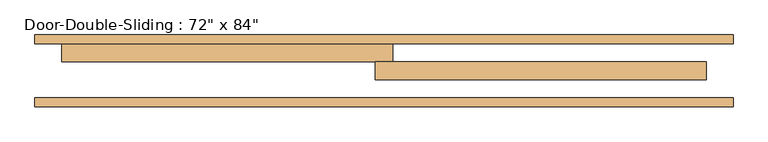
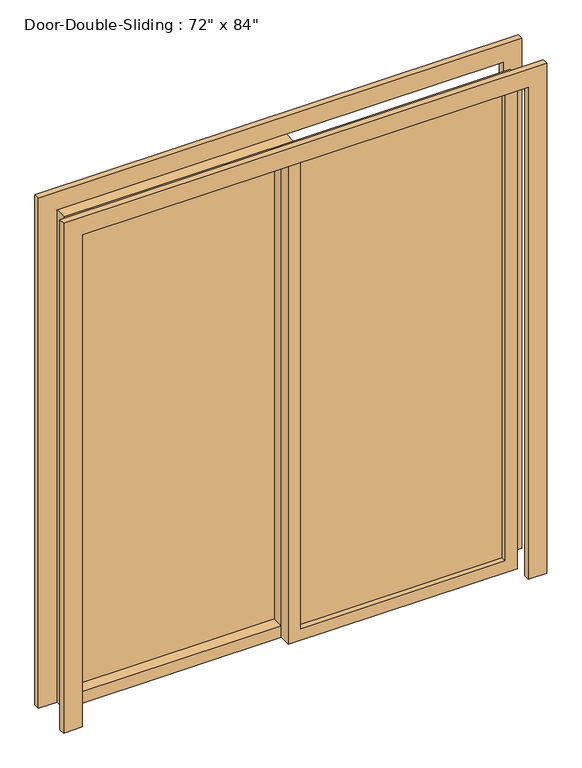
"""IFC4 building model written with IfcOpenShell, lengths in millimetres: door geometry."""

from ifc_helpers import new_model, si_unit, frame, origin, place, context, project, spatial, polyline, outline, extrude, source, transform, mapped, element, save


def door_b43bda57(model_context):
    return source(origin(), model_context, "Body", "SweptSolid", [
        extrude(outline(polyline([(0.0, -990.6), (0.0, -914.4), (2133.6, -914.4), (2133.6, 914.4), (0.0, 914.4), (0.0, 990.6), (2209.8, 990.6), (2209.8, -990.6), (0.0, -990.6)])), frame((0.0, 25.4, 0.0), z_axis=(0.0, 1.0, 0.0), x_axis=(0.0, 0.0, 1.0)), (0.0, 0.0, 1.0), 25.4),
        extrude(outline(polyline([(0.0, 990.6), (2209.8, 990.6), (2209.8, -990.6), (0.0, -990.6), (0.0, -914.4), (2133.6, -914.4), (2133.6, 914.4), (0.0, 914.4), (0.0, 990.6)])), frame((0.0, 203.2, 0.0), z_axis=(0.0, 1.0, 0.0), x_axis=(0.0, 0.0, 1.0)), (0.0, 0.0, 1.0), 25.4),
        extrude(outline(polyline([(2133.6, -25.4), (0.0, -25.4), (0.0, 914.4), (2133.6, 914.4), (2133.6, -25.4)]), holes=[polyline([(2082.8, 25.4), (2082.8, 863.6), (50.8, 863.6), (50.8, 25.4), (2082.8, 25.4)])]), frame((0.0, 101.6, 0.0), z_axis=(0.0, 1.0, 0.0), x_axis=(0.0, 0.0, 1.0)), (0.0, 0.0, 1.0), 50.8),
        extrude(outline(polyline([(2133.6, 25.4), (2133.6, -914.4), (0.0, -914.4), (0.0, 25.4), (2133.6, 25.4)]), holes=[polyline([(2082.8, -25.4), (50.8, -25.4), (50.8, -863.6), (2082.8, -863.6), (2082.8, -25.4)])]), frame((0.0, 152.4, 0.0), z_axis=(0.0, 1.0, 0.0), x_axis=(0.0, 0.0, 1.0)), (0.0, 0.0, 1.0), 50.8),
        extrude(outline(polyline([(25.4, 130.175), (863.6, 130.175), (863.6, 123.825), (25.4, 123.825), (25.4, 130.175)])), frame((0.0, 0.0, 50.8), z_axis=(0.0, 0.0, 1.0), x_axis=(1.0, 0.0, 0.0)), (0.0, 0.0, 1.0), 2032.0),
        extrude(outline(polyline([(-25.4, 200.025), (-863.6, 200.025), (-863.6, 206.375), (-25.4, 206.375), (-25.4, 200.025)])), frame((0.0, 0.0, 50.8), z_axis=(0.0, 0.0, 1.0), x_axis=(1.0, 0.0, 0.0)), (0.0, 0.0, 1.0), 2032.0),
    ])


if __name__ == "__main__":
    model = new_model("IFC4")
    model_context = context("Model", 3, world=origin())
    ifc_project = project(units=[si_unit("LENGTHUNIT", "METRE", prefix="MILLI")], contexts=[model_context])
    site = spatial("IfcSite", under=ifc_project)
    building = spatial("IfcBuilding", under=site)
    placement = place(None, origin())
    door_shape = door_b43bda57(model_context)
    element("IfcDoor", 1, ObjectType="Door-Double-Sliding : 72\" x 84\"", at=placement, inside=building, context=model_context, shape_type="MappedRepresentation", body=[
        mapped(door_shape, transform((0.0, 0.0, 0.0), x_axis=(1.0, 0.0, 0.0), y_axis=(0.0, 1.0, 0.0), z_axis=(0.0, 0.0, 1.0))),
    ])
    save(model, "model.ifc")

# Revit data of these elements
# Type "Door-Double-Sliding : 72\" x 84\""
#   Type Mark = "9"
#   Construction Type Id = "opn-d45"
#   Assembly Code = "C1020"
#   Analytic Construction = "Wood frame, double glass door "
#   Thickness = 0' - 2"
#   Thermal Resistance (R) = 1.8150 (h·ft²·°F)/BTU
#   Heat Transfer Coefficient (U) = 0.5510 BTU/(h·ft²·°F)
#   Height = 7' - 0"
#   Rail Width = 0' - 2"
#   Stiles = 0' - 2"
#   Trim Projection Ext = 0' - 1"
#   Trim Projection Int = 0' - 1"
#   Trim Width = 0' - 3"
#   Width = 6' - 0"
#   Define Thermal Properties by = 1
#   Glazing = Glass
#   Panel Material = Wood - Birch - Solid Stained Light Low Gloss
#   Trim Material = Paint - Sienna
#   Visual Light Transmittance = 0
#   Solar Heat Gain Coefficient = 0
#   Function = (empty or 0)
#   Wall Closure = (empty or 0)
# Element 1 (IfcDoor, "Door-Double-Sliding : 72\" x 84\"")
#   Materials on its faces: "Paint - Sienna", "Wood - Birch - Solid Stained Light Low Gloss", "Glass"
# Materials
#   "Glass": class "Glass", colour RGB 0 128 192, transparency 0.75, Description = "Soda Lime Glass", Cost = 0
#   "Wood - Birch - Solid Stained Light Low Gloss": class "Wood", colour RGB 210 159 95, transparency 0, Cost = 0
#   "Paint - Sienna": colour RGB 118 70 51, transparency 0, Cost = 0
